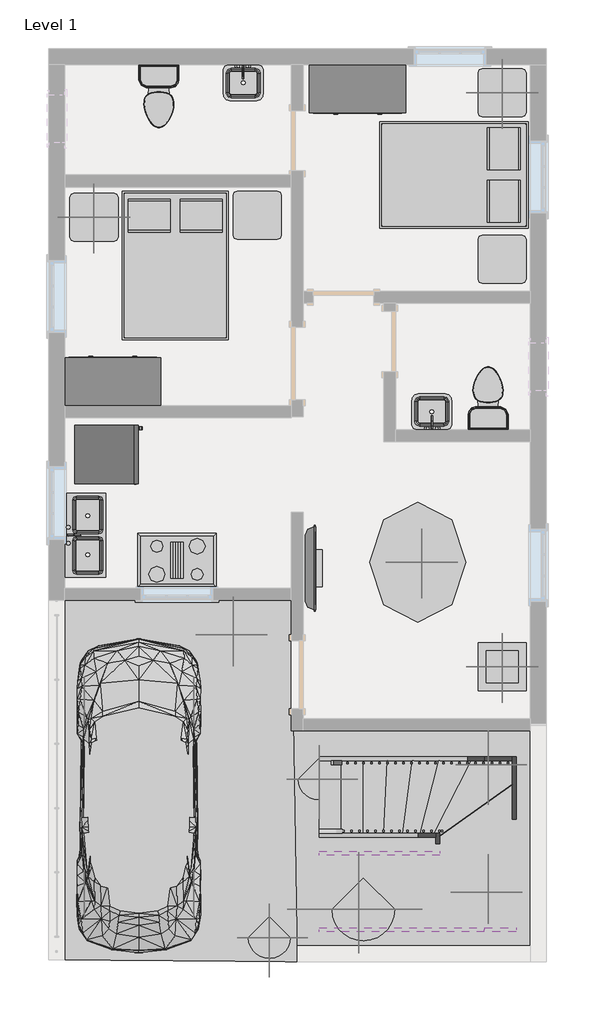
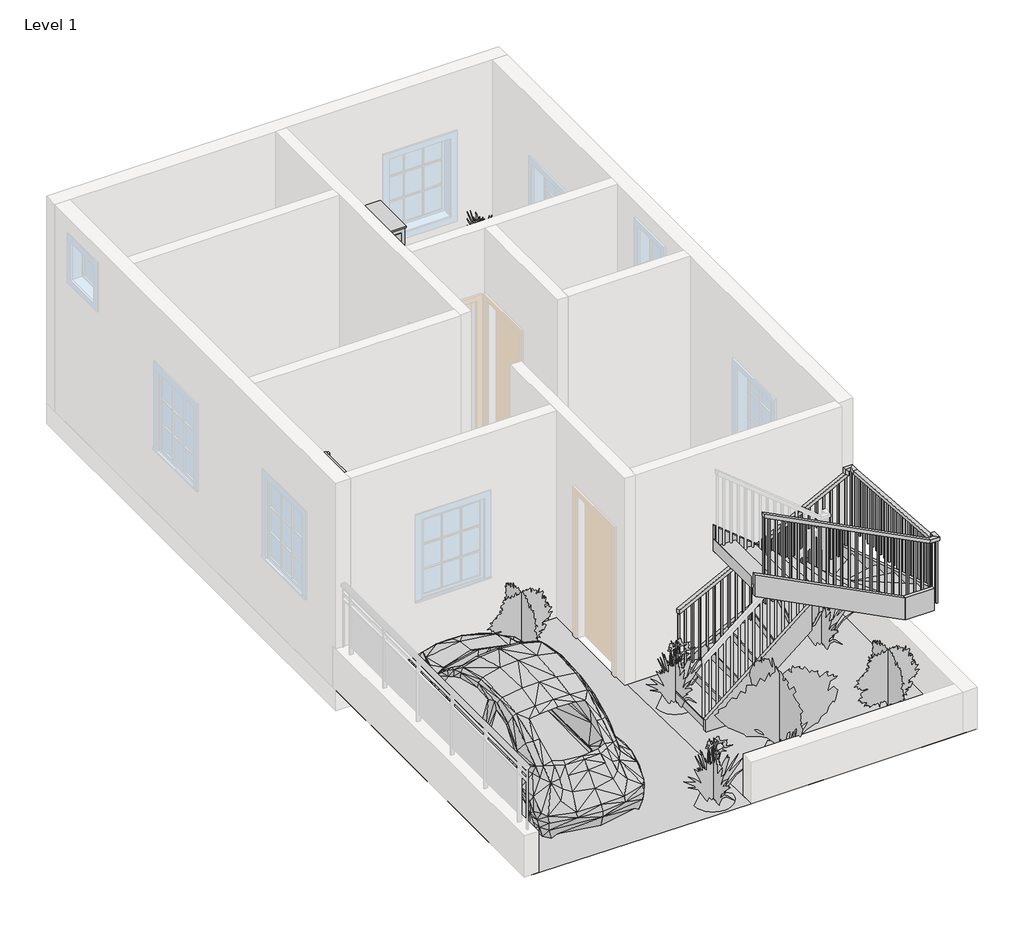
# One storey, part 2 of 2: 11 furniture elements, 10 geographic elements, 8 members, 7 flow terminals, 5 proxies, 1 railing, 1 stair flight.
"""IFC4 building model written with IfcOpenShell, lengths in millimetres."""

from ifc_helpers import new_model, si_unit, frame, origin, place, context, project, spatial, polyline, outline, extrude, faceted_brep, triangles, transform, mapped, element, save
from components import proxy_bb1e6e30, rpc_beetle_rpc_beetle_3ce7ba48, proxy_a13a33b2, flow_terminal_accce45a, flow_terminal_a53be723, flow_terminal_62a433f7, toilet_domestic_3d_toilet_domestic_3d_f7549cf7, toilet_domestic_3d_toilet_domestic_3d_183bbd19, furniture_c8abb964, furniture_2babcf72, furniture_7a3aaa4f, furniture_b5c51a22, furniture_743965d2, furniture_31d08a24, rpc_plant_tropical_55f6ff97, rpc_plant_tropical_6475341c, rpc_plant_tropical_agave_1_5_93a2a214, rpc_plant_tropical_jungle_flame_3_9c4808c2, stair_flight_9cd34823

model = new_model("IFC4")

# Units and contexts
model_context = context("Model", 3, world=origin())
ifc_project = project(units=[si_unit("LENGTHUNIT", "METRE", prefix="MILLI")], contexts=[model_context])

# Site, building, storey
site = spatial("IfcSite", under=ifc_project)
building = spatial("IfcBuilding", under=site)
storey = spatial("IfcBuildingStorey", under=building, Name="Level 1", Elevation=0.0)

# Proxies
placement = place(None, origin())
element("IfcBuildingElementProxy", 1, Name="Building Element Proxy", at=placement, inside=storey, context=model_context, shape_type="Tessellation", body=[
    triangles([(-13440.8586548, 7159.8083221, 0.0), (-10367.4590424, 7159.8083221, 0.0), (-10291.2590424, 2587.8086128, 0.0), (-13440.8586548, 2714.808419, 0.0), (-13440.8586548, 2613.2085159, 0.0)], [[4, 2, 1], [4, 3, 2], [3, 4, 5]], closed=False),
])
element("IfcBuildingElementProxy", 2, Name="Building Element Proxy", at=placement, inside=storey, context=model_context, shape_type="Tessellation", body=[
    triangles([(-7141.6588486, 5572.3087097, 0.0), (-10367.4590424, 5508.8085159, 0.0), (-10291.2590424, 2587.8086128, 0.0), (-7141.6588486, 2587.8086128, 0.0)], [[2, 3, 1], [4, 1, 3]], closed=False),
])
proxy_shape = proxy_bb1e6e30(model_context)
element("IfcBuildingElementProxy", 3, Name="Cook Top-4 Unit : 36\" x 20\"", ObjectType="Cook Top-4 Unit : 36\" x 20\"", at=placement, inside=storey, context=model_context, shape_type="MappedRepresentation", body=[
    mapped(proxy_shape, transform((-11815.2586966, 7667.8085318, 0.0), x_axis=(1.0, 0.0, 0.0), y_axis=(0.0, 1.0, 0.0), z_axis=(0.0, 0.0, 1.0))),
])
rpc_beetle_rpc_beetle_shape = rpc_beetle_rpc_beetle_3ce7ba48(model_context)
element("IfcBuildingElementProxy", 4, Name="RPC Beetle : RPC Beetle", ObjectType="RPC Beetle : RPC Beetle", at=placement, inside=storey, context=model_context, shape_type="MappedRepresentation", body=[
    mapped(rpc_beetle_rpc_beetle_shape, transform((-12297.8586966, 3451.4085318, 0.0), x_axis=(1.0, 0.0, 0.0), y_axis=(0.0, 1.0, 0.0), z_axis=(0.0, 0.0, 1.0))),
])
proxy_2_shape = proxy_a13a33b2(model_context)
element("IfcBuildingElementProxy", 5, Name="Refrigerator : 30\" x 32\" RH", ObjectType="Refrigerator : 30\" x 32\" RH", at=placement, inside=storey, context=model_context, shape_type="MappedRepresentation", body=[
    mapped(proxy_2_shape, transform((-12721.7211966, 9006.4595603, 0.0), x_axis=(0.0, 1.0000000000000002, 0.0), y_axis=(-1.0000000000000002, 0.0, 0.0), z_axis=(0.0, 0.0, 1.0))),
])

# Flow terminals
flow_terminal_shape = flow_terminal_accce45a(model_context)
element("IfcFlowTerminal", 6, ObjectType="Floor Drain - Round : 5\" Strainer - 2\" Drain", at=placement, inside=storey, context=model_context, shape_type="MappedRepresentation", body=[
    mapped(flow_terminal_shape, transform((-12907.4586966, 13738.4085318, 0.0), x_axis=(1.0, 0.0, 0.0), y_axis=(0.0, 1.0, 0.0), z_axis=(0.0, 0.0, 1.0))),
])
element("IfcFlowTerminal", 7, ObjectType="Floor Drain - Round : 5\" Strainer - 2\" Drain", at=placement, inside=storey, context=model_context, shape_type="MappedRepresentation", body=[
    mapped(flow_terminal_shape, transform((-7700.4586966, 10766.6085318, 0.0), x_axis=(1.0, 0.0, 0.0), y_axis=(0.0, 1.0, 0.0), z_axis=(0.0, 0.0, 1.0))),
])
flow_terminal_2_shape = flow_terminal_a53be723(model_context)
element("IfcFlowTerminal", 8, ObjectType="Sink Kitchen-Double : 42\" x 21\"", at=placement, inside=storey, context=model_context, shape_type="MappedRepresentation", body=[
    mapped(flow_terminal_2_shape, transform((-12981.3132954, 7969.6192912, 0.0), x_axis=(0.0, 1.0000000000000002, 0.0), y_axis=(-1.0000000000000002, 0.0, 0.0), z_axis=(0.0, 0.0, 1.0))),
])
flow_terminal_3_shape = flow_terminal_62a433f7(model_context)
element("IfcFlowTerminal", 9, ObjectType="Sink Vanity-Square : 20\" x 18\"", at=placement, inside=storey, context=model_context, shape_type="MappedRepresentation", body=[
    mapped(flow_terminal_3_shape, transform((-10992.7479371, 13761.4631306, 0.0), x_axis=(1.0, 0.0, 0.0), y_axis=(0.0, 1.0, 0.0), z_axis=(0.0, 0.0, 1.0))),
])
element("IfcFlowTerminal", 10, ObjectType="Sink Vanity-Square : 20\" x 18\"", at=placement, inside=storey, context=model_context, shape_type="MappedRepresentation", body=[
    mapped(flow_terminal_3_shape, transform((-8573.769456, 9498.9539329, 0.0), x_axis=(-1.0, 0.0, 0.0), y_axis=(0.0, -1.0, 0.0), z_axis=(0.0, 0.0, 1.0))),
])
toilet_domestic_3d_toilet_domestic_3d_shape = toilet_domestic_3d_toilet_domestic_3d_f7549cf7(model_context)
toilet_domestic_3d_toilet_domestic_3d_2_shape = toilet_domestic_3d_toilet_domestic_3d_183bbd19(model_context)
element("IfcFlowTerminal", 11, ObjectType="Toilet-Domestic-3D : Toilet-Domestic-3D", at=placement, inside=storey, context=model_context, shape_type="MappedRepresentation", body=[
    mapped(toilet_domestic_3d_toilet_domestic_3d_shape, transform((-12043.8586966, 13446.9125044, 0.0), x_axis=(1.0, 0.0, 0.0), y_axis=(0.0, 1.0, 0.0), z_axis=(0.0, 0.0, 1.0))),
    mapped(toilet_domestic_3d_toilet_domestic_3d_2_shape, transform((-12043.8586966, 13446.9125044, 0.0), x_axis=(1.0, 0.0, 0.0), y_axis=(0.0, 1.0, 0.0), z_axis=(0.0, 0.0, 1.0))),
])
element("IfcFlowTerminal", 12, ObjectType="Toilet-Domestic-3D : Toilet-Domestic-3D", at=placement, inside=storey, context=model_context, shape_type="MappedRepresentation", body=[
    mapped(toilet_domestic_3d_toilet_domestic_3d_shape, transform((-7878.2586966, 9813.5045591, 0.0), x_axis=(-1.0, 0.0, 0.0), y_axis=(0.0, -1.0, 0.0), z_axis=(0.0, 0.0, 1.0))),
    mapped(toilet_domestic_3d_toilet_domestic_3d_2_shape, transform((-7878.2586966, 9813.5045591, 0.0), x_axis=(-1.0, 0.0, 0.0), y_axis=(0.0, -1.0, 0.0), z_axis=(0.0, 0.0, 1.0))),
])

# Furniture
furniture_shape = furniture_c8abb964(model_context)
element("IfcFurniture", 13, ObjectType="Bed-Box : Double 53\" x 74\"", at=placement, inside=storey, context=model_context, shape_type="MappedRepresentation", body=[
    mapped(furniture_shape, transform((-8075.6291884, 12883.7609908, 0.0), x_axis=(0.0, -1.0000000000000004, 0.0), y_axis=(1.0000000000000004, 0.0, 0.0), z_axis=(0.0, 0.0, 1.0))),
])
element("IfcFurniture", 14, ObjectType="Bed-Box : Double 53\" x 74\"", at=placement, inside=storey, context=model_context, shape_type="MappedRepresentation", body=[
    mapped(furniture_shape, transform((-12176.6882047, 11633.9560727, 0.0), x_axis=(1.0000000000000007, 0.0, 0.0), y_axis=(0.0, 1.0000000000000007, 0.0), z_axis=(0.0, 0.0, 1.0))),
])
furniture_2_shape = furniture_2babcf72(model_context)
element("IfcFurniture", 15, ObjectType="Dresser : 48\" x 60\" x 24\"", at=placement, inside=storey, context=model_context, shape_type="MappedRepresentation", body=[
    mapped(furniture_2_shape, transform((-9260.0654367, 13999.9714858, 0.0), x_axis=(1.0, 0.0, 0.0), y_axis=(0.0, 1.0, 0.0), z_axis=(0.0, 0.0, 1.0))),
])
element("IfcFurniture", 16, ObjectType="Dresser : 48\" x 60\" x 24\"", at=placement, inside=storey, context=model_context, shape_type="MappedRepresentation", body=[
    mapped(furniture_2_shape, transform((-12897.2519564, 9565.2455777, 0.0), x_axis=(-1.0000000000000004, 0.0, 0.0), y_axis=(0.0, -1.0000000000000004, 0.0), z_axis=(0.0, 0.0, 1.0))),
])
furniture_3_shape = furniture_7a3aaa4f(model_context)
element("IfcFurniture", 17, ObjectType="TV - Flat Screen : 42\"", at=placement, inside=storey, context=model_context, shape_type="MappedRepresentation", body=[
    mapped(furniture_3_shape, transform((-10131.1200729, 7570.1530459, 914.4), x_axis=(0.0, 1.0, 0.0), y_axis=(-1.0, 0.0, 0.0), z_axis=(0.0, 0.0, 1.0))),
])
furniture_4_shape = furniture_b5c51a22(model_context)
element("IfcFurniture", 18, ObjectType="Table-Coffee : 24\" x 24\" x 24\"", at=placement, inside=storey, context=model_context, shape_type="MappedRepresentation", body=[
    mapped(furniture_4_shape, transform((-7718.7244632, 6226.3974539, 0.0), x_axis=(1.0, 0.0, 0.0), y_axis=(0.0, 1.0, 0.0), z_axis=(0.0, 0.0, 1.0))),
])
furniture_5_shape = furniture_743965d2(model_context)
element("IfcFurniture", 19, ObjectType="Table-Ellipse : 60\" x 48\"", at=placement, inside=storey, context=model_context, shape_type="MappedRepresentation", body=[
    mapped(furniture_5_shape, transform((-8767.2586966, 7642.4085318, 0.0), x_axis=(0.0, 1.0000000000000002, 0.0), y_axis=(-1.0000000000000002, 0.0, 0.0), z_axis=(0.0, 0.0, 1.0))),
])
furniture_6_shape = furniture_31d08a24(model_context)
element("IfcFurniture", 20, ObjectType="Table-End : 24\" x 24\"", at=placement, inside=storey, context=model_context, shape_type="MappedRepresentation", body=[
    mapped(furniture_6_shape, transform((-8008.9923268, 13433.6085318, 0.0), x_axis=(1.0, 0.0, 0.0), y_axis=(0.0, 1.0, 0.0), z_axis=(0.0, 0.0, 1.0))),
])
element("IfcFurniture", 21, ObjectType="Table-End : 24\" x 24\"", at=placement, inside=storey, context=model_context, shape_type="MappedRepresentation", body=[
    mapped(furniture_6_shape, transform((-8008.9923268, 11325.4085318, 0.0), x_axis=(1.0, 0.0, 0.0), y_axis=(0.0, 1.0, 0.0), z_axis=(0.0, 0.0, 1.0))),
])
element("IfcFurniture", 22, ObjectType="Table-End : 24\" x 24\"", at=placement, inside=storey, context=model_context, shape_type="MappedRepresentation", body=[
    mapped(furniture_6_shape, transform((-11107.7923268, 11882.1265645, 0.0), x_axis=(1.0, 0.0, 0.0), y_axis=(0.0, 1.0, 0.0), z_axis=(0.0, 0.0, 1.0))),
])
element("IfcFurniture", 23, ObjectType="Table-End : 24\" x 24\"", at=placement, inside=storey, context=model_context, shape_type="MappedRepresentation", body=[
    mapped(furniture_6_shape, transform((-13174.769376, 11856.7265645, 0.0), x_axis=(1.0, 0.0, 0.0), y_axis=(0.0, 1.0, 0.0), z_axis=(0.0, 0.0, 1.0))),
])

# Geographic elements
rpc_plant_tropical_shape = rpc_plant_tropical_55f6ff97(model_context)
element("IfcGeographicElement", 24, ObjectType="RPC Plant - Tropical", at=placement, inside=storey, context=model_context, shape_type="MappedRepresentation", body=[
    mapped(rpc_plant_tropical_shape, transform((-10646.8586966, 2892.6085318, 0.0), x_axis=(1.0, 0.0, 0.0), y_axis=(0.0, 1.0, 0.0), z_axis=(0.0, 0.0, 1.0))),
])
element("IfcGeographicElement", 25, ObjectType="RPC Plant - Tropical", at=placement, inside=storey, context=model_context, shape_type="MappedRepresentation", body=[
    mapped(rpc_plant_tropical_shape, transform((-7878.2586966, 5077.0085318, 0.0), x_axis=(1.0, 0.0, 0.0), y_axis=(0.0, 1.0, 0.0), z_axis=(0.0, 0.0, 1.0))),
])
element("IfcGeographicElement", 26, ObjectType="RPC Plant - Tropical", at=placement, inside=storey, context=model_context, shape_type="MappedRepresentation", body=[
    mapped(rpc_plant_tropical_shape, transform((-10015.5903884, 4899.2085318, 0.0), x_axis=(1.0, 0.0, 0.0), y_axis=(0.0, 1.0, 0.0), z_axis=(0.0, 0.0, 1.0))),
])
rpc_plant_tropical_2_shape = rpc_plant_tropical_6475341c(model_context)
element("IfcGeographicElement", 27, ObjectType="RPC Plant - Tropical", at=placement, inside=storey, context=model_context, shape_type="MappedRepresentation", body=[
    mapped(rpc_plant_tropical_2_shape, transform((-9456.7903884, 3248.2085318, 0.0), x_axis=(1.0, 0.0, 0.0), y_axis=(0.0, 1.0, 0.0), z_axis=(0.0, 0.0, 1.0))),
])
rpc_plant_tropical_agave_1_5_shape = rpc_plant_tropical_agave_1_5_93a2a214(model_context)
element("IfcGeographicElement", 28, ObjectType="RPC Plant - Tropical : Agave - 1.5'", at=placement, inside=storey, context=model_context, shape_type="MappedRepresentation", body=[
    mapped(rpc_plant_tropical_agave_1_5_shape, transform((-7700.4586966, 13586.0085318, 609.6), x_axis=(1.0, 0.0, 0.0), y_axis=(0.0, 1.0, 0.0), z_axis=(0.0, 0.0, 1.0))),
])
element("IfcGeographicElement", 29, ObjectType="RPC Plant - Tropical : Agave - 1.5'", at=placement, inside=storey, context=model_context, shape_type="MappedRepresentation", body=[
    mapped(rpc_plant_tropical_agave_1_5_shape, transform((-12866.2357457, 12009.1265645, 609.6), x_axis=(1.0, 0.0, 0.0), y_axis=(0.0, 1.0, 0.0), z_axis=(0.0, 0.0, 1.0))),
])
element("IfcGeographicElement", 30, ObjectType="RPC Plant - Tropical : Agave - 1.5'", at=placement, inside=storey, context=model_context, shape_type="MappedRepresentation", body=[
    mapped(rpc_plant_tropical_agave_1_5_shape, transform((-7700.4586966, 6321.6085318, 609.6), x_axis=(1.0, 0.0, 0.0), y_axis=(0.0, 1.0, 0.0), z_axis=(0.0, 0.0, 1.0))),
])
element("IfcGeographicElement", 31, ObjectType="RPC Plant - Tropical : Agave - 1.5'", at=placement, inside=storey, context=model_context, shape_type="MappedRepresentation", body=[
    mapped(rpc_plant_tropical_agave_1_5_shape, transform((-8716.4586966, 7642.4085318, 762.0), x_axis=(1.0, 0.0, 0.0), y_axis=(0.0, 1.0, 0.0), z_axis=(0.0, 0.0, 1.0))),
])
rpc_plant_tropical_jungle_flame_3_shape = rpc_plant_tropical_jungle_flame_3_9c4808c2(model_context)
element("IfcGeographicElement", 32, ObjectType="RPC Plant - Tropical : Jungle Flame - 3'", at=placement, inside=storey, context=model_context, shape_type="MappedRepresentation", body=[
    mapped(rpc_plant_tropical_jungle_flame_3_shape, transform((-11104.0586966, 6728.0085318, 0.0), x_axis=(1.0, 0.0, 0.0), y_axis=(0.0, 1.0, 0.0), z_axis=(0.0, 0.0, 1.0))),
])
element("IfcGeographicElement", 33, ObjectType="RPC Plant - Tropical : Jungle Flame - 3'", at=placement, inside=storey, context=model_context, shape_type="MappedRepresentation", body=[
    mapped(rpc_plant_tropical_jungle_flame_3_shape, transform((-7878.2586966, 3467.7118501, 0.0), x_axis=(1.0, 0.0, 0.0), y_axis=(0.0, 1.0, 0.0), z_axis=(0.0, 0.0, 1.0))),
])

# Members
element("IfcMember", 34, ObjectType="Stringer - 2\" Width", at=placement, inside=storey, context=model_context, shape_type="SweptSolid", body=[
    extrude(outline(polyline([(229.639954, -10015.5903884), (0.0, -10015.5903884), (0.0, -9795.8280709), (962.500629, -7928.1731967), (1305.3956453, -7928.1731967), (229.639954, -10015.5903884)])), frame((0.0, 5127.8085318, 0.0), z_axis=(0.0, 1.0, 0.0), x_axis=(0.0, 0.0, 1.0)), (0.0, 0.0, 1.0), 50.8),
])
element("IfcMember", 35, ObjectType="Stringer - 2\" Width", at=placement, inside=storey, context=model_context, shape_type="SweptSolid", body=[
    extrude(outline(polyline([(-7928.1731967, 5127.8085318), (-7928.1731967, 5178.6085318), (-7573.4586966, 5178.6085318), (-7573.4586966, 5127.8085318), (-7928.1731967, 5127.8085318)])), frame((0.0, 0.0, 962.500629), z_axis=(0.0, 0.0, 1.0), x_axis=(1.0, 0.0, 0.0)), (0.0, 0.0, 1.0), 342.8950162),
])
element("IfcMember", 36, ObjectType="Stringer - 2\" Width", at=placement, inside=storey, context=model_context, shape_type="SweptSolid", body=[
    extrude(outline(polyline([(5178.6085318, 1289.0952212), (5178.6085318, 1000.5956453), (5009.0860488, 1000.5956453), (3019.6085318, 1638.9682298), (3019.6085318, 1969.9972697), (3056.588649, 1969.9972697), (5178.6085318, 1289.0952212)])), frame((-7573.4586966, 0.0, 0.0), z_axis=(1.0, 0.0, 0.0), x_axis=(0.0, 1.0, 0.0)), (0.0, 0.0, 1.0), 50.8),
])
element("IfcMember", 37, ObjectType="Stringer - 2\" Width", at=placement, inside=storey, context=model_context, shape_type="SweptSolid", body=[
    extrude(outline(polyline([(-7522.6586966, 3019.6085318), (-7522.6586966, 2968.8085318), (-7928.1731967, 2968.8085318), (-7928.1731967, 3019.6085318), (-7522.6586966, 3019.6085318)])), frame((0.0, 0.0, 1649.8904473), z_axis=(0.0, 0.0, 1.0), x_axis=(1.0, 0.0, 0.0)), (0.0, 0.0, 1.0), 320.1068224),
])
element("IfcMember", 38, ObjectType="Stringer - 2\" Width", at=placement, inside=storey, context=model_context, shape_type="SweptSolid", body=[
    extrude(outline(polyline([(1649.8904473, -7928.1731967), (1969.9972697, -7928.1731967), (3045.7529609, -10015.5903884), (2725.6461385, -10015.5903884), (1649.8904473, -7928.1731967)])), frame((0.0, 2968.8085318, 0.0), z_axis=(0.0, 1.0, 0.0), x_axis=(0.0, 0.0, 1.0)), (0.0, 0.0, 1.0), 50.8),
])
element("IfcMember", 39, ObjectType="Stringer - 2\" Width", at=placement, inside=storey, context=model_context, shape_type="SweptSolid", body=[
    extrude(outline(polyline([(176.1764461, -10015.5903884), (0.0, -10015.5903884), (0.0, -9749.3287439), (987.1410923, -8538.6586966), (1380.418648, -8538.6586966), (176.1764461, -10015.5903884)])), frame((0.0, 4162.6085318, 0.0), z_axis=(0.0, 1.0, 0.0), x_axis=(0.0, 0.0, 1.0)), (0.0, 0.0, 1.0), 50.8),
])
element("IfcMember", 40, ObjectType="Stringer - 2\" Width", at=placement, inside=storey, context=model_context, shape_type="SweptSolid", body=[
    extrude(outline(polyline([(4213.4085318, 1573.2682978), (4213.4085318, 1028.5617647), (4179.1663144, 1028.5617647), (3984.8085318, 1360.465107), (3984.8085318, 1926.1409689), (4006.7714143, 1926.1409689), (4213.4085318, 1573.2682978)])), frame((-8538.6586966, 0.0, 0.0), z_axis=(1.0, 0.0, 0.0), x_axis=(0.0, 1.0, 0.0)), (0.0, 0.0, 1.0), 50.8),
])
element("IfcMember", 41, ObjectType="Stringer - 2\" Width", at=placement, inside=storey, context=model_context, shape_type="SweptSolid", body=[
    extrude(outline(polyline([(1532.8634131, -8487.8586966), (1926.1409689, -8487.8586966), (3171.8038432, -10015.5903884), (2778.5262875, -10015.5903884), (1532.8634131, -8487.8586966)])), frame((0.0, 3934.0085318, 0.0), z_axis=(0.0, 1.0, 0.0), x_axis=(0.0, 0.0, 1.0)), (0.0, 0.0, 1.0), 50.8),
])

# Railing
element("IfcRailing", 42, ObjectType="Handrail - Rectangular", at=placement, inside=storey, context=model_context, shape_type="SolidModel", body=[
    faceted_brep([(-9863.1903884, 5127.8085318, 1187.6168978), (-9863.1903884, 5127.8085318, 1130.4677284), (-9863.1903884, 5077.0085318, 1130.4677284), (-9863.1903884, 5077.0085318, 1187.6168978), (-7548.0586966, 5127.8085318, 2380.7258284), (-7497.2586966, 5127.8085318, 2349.7565666), (-7497.2586966, 5077.0085318, 2349.7565666), (-7548.0586966, 5077.0085318, 2380.7258284), (-7421.0586966, 4998.958193, 2404.6395816), (-7421.0586966, 5000.8085318, 2455.4395816), (-7421.0586966, 3146.6085318, 2590.6937517), (-7421.0586966, 3095.8085318, 2543.4643729), (-7471.8586966, 4998.958193, 2404.6395816), (-7471.8586966, 3095.8085318, 2543.4643729), (-7471.8586966, 5000.8085318, 2455.4395816), (-7471.8586966, 3146.6085318, 2590.6937517), (-9863.1903884, 3019.6085318, 3858.5164356), (-9863.1903884, 3070.4085318, 3858.5164356), (-9863.1903884, 3070.4085318, 3801.3672662), (-9863.1903884, 3019.6085318, 3801.3672662), (-7560.3787478, 3019.6085318, 2614.6075049), (-7548.0586966, 3019.6085318, 2665.4075049), (-7560.3787478, 3070.4085318, 2614.6075049), (-7548.0586966, 3070.4085318, 2665.4075049), (-7548.0586966, 5127.8085318, 2455.4395816), (-7497.2586966, 5127.8085318, 2404.6395816), (-7497.2586966, 5077.0085318, 2404.6395816), (-7548.0586966, 5077.0085318, 2455.4395816), (-7421.0586966, 5127.8085318, 2455.4395816), (-7421.0586966, 5127.8085318, 2404.6395816), (-7471.8586966, 5077.0085318, 2404.6395816), (-7471.8586966, 5077.0085318, 2455.4395816), (-7421.0586966, 3146.6085318, 2665.4075049), (-7421.0586966, 3095.8085318, 2614.6075049), (-7471.8586966, 3095.8085318, 2614.6075049), (-7471.8586966, 3146.6085318, 2665.4075049), (-7421.0586966, 3019.6085318, 2665.4075049), (-7421.0586966, 3019.6085318, 2614.6075049), (-7471.8586966, 3070.4085318, 2614.6075049), (-7471.8586966, 3070.4085318, 2665.4075049)], [[[0, 1, 2, 3]], [[1, 0, 4, 5]], [[2, 1, 5, 6]], [[3, 2, 6, 7]], [[0, 3, 7, 4]], [[8, 9, 10, 11]], [[12, 8, 11, 13]], [[14, 12, 13, 15]], [[9, 14, 15, 10]], [[16, 17, 18, 19]], [[20, 21, 16, 19]], [[22, 20, 19, 18]], [[23, 22, 18, 17]], [[21, 23, 17, 16]], [[5, 4, 24, 25]], [[6, 5, 25, 26]], [[7, 6, 26, 27]], [[4, 7, 27, 24]], [[25, 24, 28, 29]], [[26, 25, 29, 30]], [[27, 26, 30, 31]], [[24, 27, 31, 28]], [[29, 28, 9, 8]], [[30, 29, 8, 12]], [[31, 30, 12, 14]], [[28, 31, 14, 9]], [[11, 10, 32, 33]], [[13, 11, 33, 34]], [[15, 13, 34, 35]], [[10, 15, 35, 32]], [[33, 32, 36, 37]], [[34, 33, 37, 38]], [[35, 34, 38, 39]], [[32, 35, 39, 36]], [[37, 36, 21, 20]], [[38, 37, 20, 22]], [[39, 38, 22, 23]], [[36, 39, 23, 21]]]),
    extrude(outline(polyline([(3765.0830008, -9792.7836966), (2878.6666667, -9792.7836966), (2878.6666667, -9773.7336966), (3755.2655354, -9773.7336966), (3765.0830008, -9792.7836966)])), frame((0.0, 3035.4835318, 0.0), z_axis=(0.0, 1.0, 0.0), x_axis=(0.0, 0.0, 1.0)), (0.0, 0.0, 1.0), 19.05),
    extrude(outline(polyline([(3712.7231856, -9691.1836966), (2709.3333333, -9691.1836966), (2709.3333333, -9672.1336966), (3702.9057203, -9672.1336966), (3712.7231856, -9691.1836966)])), frame((0.0, 3035.4835318, 0.0), z_axis=(0.0, 1.0, 0.0), x_axis=(0.0, 0.0, 1.0)), (0.0, 0.0, 1.0), 19.05),
    extrude(outline(polyline([(3660.3633705, -9589.5836966), (2709.3333333, -9589.5836966), (2709.3333333, -9570.5336966), (3650.5459052, -9570.5336966), (3660.3633705, -9589.5836966)])), frame((0.0, 3035.4835318, 0.0), z_axis=(0.0, 1.0, 0.0), x_axis=(0.0, 0.0, 1.0)), (0.0, 0.0, 1.0), 19.05),
    extrude(outline(polyline([(3608.0035554, -9487.9836966), (2709.3333333, -9487.9836966), (2709.3333333, -9468.9336966), (3598.1860901, -9468.9336966), (3608.0035554, -9487.9836966)])), frame((0.0, 3035.4835318, 0.0), z_axis=(0.0, 1.0, 0.0), x_axis=(0.0, 0.0, 1.0)), (0.0, 0.0, 1.0), 19.05),
    extrude(outline(polyline([(3555.6437403, -9386.3836966), (2540.0, -9386.3836966), (2540.0, -9367.3336966), (3545.826275, -9367.3336966), (3555.6437403, -9386.3836966)])), frame((0.0, 3035.4835318, 0.0), z_axis=(0.0, 1.0, 0.0), x_axis=(0.0, 0.0, 1.0)), (0.0, 0.0, 1.0), 19.05),
    extrude(outline(polyline([(3503.2839252, -9284.7836966), (2540.0, -9284.7836966), (2540.0, -9265.7336966), (3493.4664598, -9265.7336966), (3503.2839252, -9284.7836966)])), frame((0.0, 3035.4835318, 0.0), z_axis=(0.0, 1.0, 0.0), x_axis=(0.0, 0.0, 1.0)), (0.0, 0.0, 1.0), 19.05),
    extrude(outline(polyline([(3450.9241101, -9183.1836966), (2540.0, -9183.1836966), (2540.0, -9164.1336966), (3441.1066447, -9164.1336966), (3450.9241101, -9183.1836966)])), frame((0.0, 3035.4835318, 0.0), z_axis=(0.0, 1.0, 0.0), x_axis=(0.0, 0.0, 1.0)), (0.0, 0.0, 1.0), 19.05),
    extrude(outline(polyline([(3398.5642949, -9081.5836966), (2370.6666667, -9081.5836966), (2370.6666667, -9062.5336966), (3388.7468296, -9062.5336966), (3398.5642949, -9081.5836966)])), frame((0.0, 3035.4835318, 0.0), z_axis=(0.0, 1.0, 0.0), x_axis=(0.0, 0.0, 1.0)), (0.0, 0.0, 1.0), 19.05),
    extrude(outline(polyline([(3346.2044798, -8979.9836966), (2370.6666667, -8979.9836966), (2370.6666667, -8960.9336966), (3336.3870145, -8960.9336966), (3346.2044798, -8979.9836966)])), frame((0.0, 3035.4835318, 0.0), z_axis=(0.0, 1.0, 0.0), x_axis=(0.0, 0.0, 1.0)), (0.0, 0.0, 1.0), 19.05),
    extrude(outline(polyline([(3293.8446647, -8878.3836966), (2370.6666667, -8878.3836966), (2370.6666667, -8859.3336966), (3284.0271994, -8859.3336966), (3293.8446647, -8878.3836966)])), frame((0.0, 3035.4835318, 0.0), z_axis=(0.0, 1.0, 0.0), x_axis=(0.0, 0.0, 1.0)), (0.0, 0.0, 1.0), 19.05),
    extrude(outline(polyline([(3241.4848496, -8776.7836966), (2201.3333333, -8776.7836966), (2201.3333333, -8757.7336966), (3231.6673843, -8757.7336966), (3241.4848496, -8776.7836966)])), frame((0.0, 3035.4835318, 0.0), z_axis=(0.0, 1.0, 0.0), x_axis=(0.0, 0.0, 1.0)), (0.0, 0.0, 1.0), 19.05),
    extrude(outline(polyline([(3189.1250345, -8675.1836966), (2201.3333333, -8675.1836966), (2201.3333333, -8656.1336966), (3179.3075691, -8656.1336966), (3189.1250345, -8675.1836966)])), frame((0.0, 3035.4835318, 0.0), z_axis=(0.0, 1.0, 0.0), x_axis=(0.0, 0.0, 1.0)), (0.0, 0.0, 1.0), 19.05),
    extrude(outline(polyline([(3136.7652194, -8573.5836966), (2201.3333333, -8573.5836966), (2201.3333333, -8554.5336966), (3126.947754, -8554.5336966), (3136.7652194, -8573.5836966)])), frame((0.0, 3035.4835318, 0.0), z_axis=(0.0, 1.0, 0.0), x_axis=(0.0, 0.0, 1.0)), (0.0, 0.0, 1.0), 19.05),
    extrude(outline(polyline([(3084.4054042, -8471.9836966), (2032.0, -8471.9836966), (2032.0, -8452.9336966), (3074.5879389, -8452.9336966), (3084.4054042, -8471.9836966)])), frame((0.0, 3035.4835318, 0.0), z_axis=(0.0, 1.0, 0.0), x_axis=(0.0, 0.0, 1.0)), (0.0, 0.0, 1.0), 19.05),
    extrude(outline(polyline([(3032.0455891, -8370.3836966), (2032.0, -8370.3836966), (2032.0, -8351.3336966), (3022.2281238, -8351.3336966), (3032.0455891, -8370.3836966)])), frame((0.0, 3035.4835318, 0.0), z_axis=(0.0, 1.0, 0.0), x_axis=(0.0, 0.0, 1.0)), (0.0, 0.0, 1.0), 19.05),
    extrude(outline(polyline([(2979.685774, -8268.7836966), (2032.0, -8268.7836966), (2032.0, -8249.7336966), (2969.8683087, -8249.7336966), (2979.685774, -8268.7836966)])), frame((0.0, 3035.4835318, 0.0), z_axis=(0.0, 1.0, 0.0), x_axis=(0.0, 0.0, 1.0)), (0.0, 0.0, 1.0), 19.05),
    extrude(outline(polyline([(2927.3259589, -8167.1836966), (2032.0, -8167.1836966), (2032.0, -8148.1336966), (2917.5084936, -8148.1336966), (2927.3259589, -8167.1836966)])), frame((0.0, 3035.4835318, 0.0), z_axis=(0.0, 1.0, 0.0), x_axis=(0.0, 0.0, 1.0)), (0.0, 0.0, 1.0), 19.05),
    extrude(outline(polyline([(2874.9661438, -8065.5836966), (1862.6666667, -8065.5836966), (1862.6666667, -8046.5336966), (2865.1486784, -8046.5336966), (2874.9661438, -8065.5836966)])), frame((0.0, 3035.4835318, 0.0), z_axis=(0.0, 1.0, 0.0), x_axis=(0.0, 0.0, 1.0)), (0.0, 0.0, 1.0), 19.05),
    extrude(outline(polyline([(2822.6063287, -7963.9836966), (1862.6666667, -7963.9836966), (1862.6666667, -7944.9336966), (2812.7888633, -7944.9336966), (2822.6063287, -7963.9836966)])), frame((0.0, 3035.4835318, 0.0), z_axis=(0.0, 1.0, 0.0), x_axis=(0.0, 0.0, 1.0)), (0.0, 0.0, 1.0), 19.05),
    extrude(outline(polyline([(2770.2465135, -7862.3836966), (1862.6666667, -7862.3836966), (1862.6666667, -7843.3336966), (2760.4290482, -7843.3336966), (2770.2465135, -7862.3836966)])), frame((0.0, 3035.4835318, 0.0), z_axis=(0.0, 1.0, 0.0), x_axis=(0.0, 0.0, 1.0)), (0.0, 0.0, 1.0), 19.05),
    extrude(outline(polyline([(2717.8866984, -7760.7836966), (1862.6666667, -7760.7836966), (1862.6666667, -7741.7336966), (2708.0692331, -7741.7336966), (2717.8866984, -7760.7836966)])), frame((0.0, 3035.4835318, 0.0), z_axis=(0.0, 1.0, 0.0), x_axis=(0.0, 0.0, 1.0)), (0.0, 0.0, 1.0), 19.05),
    extrude(outline(polyline([(2665.5268833, -7659.1836966), (1862.6666667, -7659.1836966), (1862.6666667, -7640.1336966), (2655.709418, -7640.1336966), (2665.5268833, -7659.1836966)])), frame((0.0, 3035.4835318, 0.0), z_axis=(0.0, 1.0, 0.0), x_axis=(0.0, 0.0, 1.0)), (0.0, 0.0, 1.0), 19.05),
    extrude(outline(polyline([(-7538.5336966, 3035.4835318), (-7557.5836966, 3035.4835318), (-7557.5836966, 3054.5335318), (-7538.5336966, 3054.5335318), (-7538.5336966, 3035.4835318)])), frame((0.0, 0.0, 1969.9972697), z_axis=(0.0, 0.0, 1.0), x_axis=(1.0, 0.0, 0.0)), (0.0, 0.0, 1.0), 644.6102352),
    extrude(outline(polyline([(-7436.9336966, 3079.9335318), (-7436.9336966, 3060.8835318), (-7455.9836966, 3060.8835318), (-7455.9836966, 3079.9335318), (-7436.9336966, 3079.9335318)])), frame((0.0, 0.0, 1681.8521423), z_axis=(0.0, 0.0, 1.0), x_axis=(1.0, 0.0, 0.0)), (0.0, 0.0, 1.0), 932.7553626),
    extrude(outline(polyline([(3181.5335318, 2537.2111836), (3181.5335318, 1674.4409549), (3162.4835318, 1674.4409549), (3162.4835318, 2538.6007812), (3181.5335318, 2537.2111836)])), frame((-7455.9836966, 0.0, 0.0), z_axis=(1.0, 0.0, 0.0), x_axis=(0.0, 1.0, 0.0)), (0.0, 0.0, 1.0), 19.05),
    extrude(outline(polyline([(3283.1335318, 2529.7999962), (3283.1335318, 1667.0297675), (3264.0835318, 1667.0297675), (3264.0835318, 2531.1895938), (3283.1335318, 2529.7999962)])), frame((-7455.9836966, 0.0, 0.0), z_axis=(1.0, 0.0, 0.0), x_axis=(0.0, 1.0, 0.0)), (0.0, 0.0, 1.0), 19.05),
    extrude(outline(polyline([(3384.7335318, 2522.3888087), (3384.7335318, 1659.6185801), (3365.6835318, 1659.6185801), (3365.6835318, 2523.7784064), (3384.7335318, 2522.3888087)])), frame((-7455.9836966, 0.0, 0.0), z_axis=(1.0, 0.0, 0.0), x_axis=(0.0, 1.0, 0.0)), (0.0, 0.0, 1.0), 19.05),
    extrude(outline(polyline([(3486.3335318, 2514.9776213), (3486.3335318, 1652.2073927), (3467.2835318, 1652.2073927), (3467.2835318, 2516.367219), (3486.3335318, 2514.9776213)])), frame((-7455.9836966, 0.0, 0.0), z_axis=(1.0, 0.0, 0.0), x_axis=(0.0, 1.0, 0.0)), (0.0, 0.0, 1.0), 19.05),
    extrude(outline(polyline([(3587.9335318, 2507.5664339), (3587.9335318, 1644.7962053), (3568.8835318, 1644.7962053), (3568.8835318, 2508.9560316), (3587.9335318, 2507.5664339)])), frame((-7455.9836966, 0.0, 0.0), z_axis=(1.0, 0.0, 0.0), x_axis=(0.0, 1.0, 0.0)), (0.0, 0.0, 1.0), 19.05),
    extrude(outline(polyline([(3689.5335318, 2500.1552465), (3689.5335318, 1637.3850179), (3670.4835318, 1637.3850179), (3670.4835318, 2501.5448442), (3689.5335318, 2500.1552465)])), frame((-7455.9836966, 0.0, 0.0), z_axis=(1.0, 0.0, 0.0), x_axis=(0.0, 1.0, 0.0)), (0.0, 0.0, 1.0), 19.05),
    extrude(outline(polyline([(3791.1335318, 2492.7440591), (3791.1335318, 1629.9738305), (3772.0835318, 1629.9738305), (3772.0835318, 2494.1336568), (3791.1335318, 2492.7440591)])), frame((-7455.9836966, 0.0, 0.0), z_axis=(1.0, 0.0, 0.0), x_axis=(0.0, 1.0, 0.0)), (0.0, 0.0, 1.0), 19.05),
    extrude(outline(polyline([(3892.7335318, 2485.3328717), (3892.7335318, 1622.5626431), (3873.6835318, 1622.5626431), (3873.6835318, 2486.7224694), (3892.7335318, 2485.3328717)])), frame((-7455.9836966, 0.0, 0.0), z_axis=(1.0, 0.0, 0.0), x_axis=(0.0, 1.0, 0.0)), (0.0, 0.0, 1.0), 19.05),
    extrude(outline(polyline([(3994.3335318, 2477.9216843), (3994.3335318, 1615.1514556), (3975.2835318, 1615.1514556), (3975.2835318, 2479.311282), (3994.3335318, 2477.9216843)])), frame((-7455.9836966, 0.0, 0.0), z_axis=(1.0, 0.0, 0.0), x_axis=(0.0, 1.0, 0.0)), (0.0, 0.0, 1.0), 19.05),
    extrude(outline(polyline([(4095.9335318, 2470.5104969), (4095.9335318, 1607.7402682), (4076.8835318, 1607.7402682), (4076.8835318, 2471.9000945), (4095.9335318, 2470.5104969)])), frame((-7455.9836966, 0.0, 0.0), z_axis=(1.0, 0.0, 0.0), x_axis=(0.0, 1.0, 0.0)), (0.0, 0.0, 1.0), 19.05),
    extrude(outline(polyline([(4197.5335318, 2463.0993095), (4197.5335318, 1600.3290808), (4178.4835318, 1600.3290808), (4178.4835318, 2464.4889071), (4197.5335318, 2463.0993095)])), frame((-7455.9836966, 0.0, 0.0), z_axis=(1.0, 0.0, 0.0), x_axis=(0.0, 1.0, 0.0)), (0.0, 0.0, 1.0), 19.05),
    extrude(outline(polyline([(4299.1335318, 2455.6881221), (4299.1335318, 1592.9178934), (4280.0835318, 1592.9178934), (4280.0835318, 2457.0777197), (4299.1335318, 2455.6881221)])), frame((-7455.9836966, 0.0, 0.0), z_axis=(1.0, 0.0, 0.0), x_axis=(0.0, 1.0, 0.0)), (0.0, 0.0, 1.0), 19.05),
    extrude(outline(polyline([(4400.7335318, 2448.2769347), (4400.7335318, 1585.506706), (4381.6835318, 1585.506706), (4381.6835318, 2449.6665323), (4400.7335318, 2448.2769347)])), frame((-7455.9836966, 0.0, 0.0), z_axis=(1.0, 0.0, 0.0), x_axis=(0.0, 1.0, 0.0)), (0.0, 0.0, 1.0), 19.05),
    extrude(outline(polyline([(4502.3335318, 2440.8657473), (4502.3335318, 1578.0955186), (4483.2835318, 1578.0955186), (4483.2835318, 2442.2553449), (4502.3335318, 2440.8657473)])), frame((-7455.9836966, 0.0, 0.0), z_axis=(1.0, 0.0, 0.0), x_axis=(0.0, 1.0, 0.0)), (0.0, 0.0, 1.0), 19.05),
    extrude(outline(polyline([(4603.9335318, 2433.4545599), (4603.9335318, 1570.6843312), (4584.8835318, 1570.6843312), (4584.8835318, 2434.8441575), (4603.9335318, 2433.4545599)])), frame((-7455.9836966, 0.0, 0.0), z_axis=(1.0, 0.0, 0.0), x_axis=(0.0, 1.0, 0.0)), (0.0, 0.0, 1.0), 19.05),
    extrude(outline(polyline([(4705.5335318, 2426.0433725), (4705.5335318, 1563.2731438), (4686.4835318, 1563.2731438), (4686.4835318, 2427.4329701), (4705.5335318, 2426.0433725)])), frame((-7455.9836966, 0.0, 0.0), z_axis=(1.0, 0.0, 0.0), x_axis=(0.0, 1.0, 0.0)), (0.0, 0.0, 1.0), 19.05),
    extrude(outline(polyline([(4807.1335318, 2418.6321851), (4807.1335318, 1555.8619564), (4788.0835318, 1555.8619564), (4788.0835318, 2420.0217827), (4807.1335318, 2418.6321851)])), frame((-7455.9836966, 0.0, 0.0), z_axis=(1.0, 0.0, 0.0), x_axis=(0.0, 1.0, 0.0)), (0.0, 0.0, 1.0), 19.05),
    extrude(outline(polyline([(4908.7335318, 2411.2209977), (4908.7335318, 1548.450769), (4889.6835318, 1548.450769), (4889.6835318, 2412.6105953), (4908.7335318, 2411.2209977)])), frame((-7455.9836966, 0.0, 0.0), z_axis=(1.0, 0.0, 0.0), x_axis=(0.0, 1.0, 0.0)), (0.0, 0.0, 1.0), 19.05),
    extrude(outline(polyline([(-7436.9336966, 5010.3335318), (-7436.9336966, 4991.2835318), (-7455.9836966, 4991.2835318), (-7455.9836966, 5010.3335318), (-7436.9336966, 5010.3335318)])), frame((0.0, 0.0, 1541.0395816), z_axis=(0.0, 0.0, 1.0), x_axis=(1.0, 0.0, 0.0)), (0.0, 0.0, 1.0), 863.6),
    extrude(outline(polyline([(2329.8347434, -7535.9153884), (1310.4895278, -7535.9153884), (1316.6021868, -7516.8653884), (2339.6522087, -7516.8653884), (2329.8347434, -7535.9153884)])), frame((0.0, 5092.8835318, 0.0), z_axis=(0.0, 1.0, 0.0), x_axis=(0.0, 0.0, 1.0)), (0.0, 0.0, 1.0), 19.05),
    extrude(outline(polyline([(2277.4749283, -7637.5153884), (1185.3333333, -7637.5153884), (1185.3333333, -7618.4653884), (2287.2923936, -7618.4653884), (2277.4749283, -7637.5153884)])), frame((0.0, 5092.8835318, 0.0), z_axis=(0.0, 1.0, 0.0), x_axis=(0.0, 0.0, 1.0)), (0.0, 0.0, 1.0), 19.05),
    extrude(outline(polyline([(2225.1151132, -7739.1153884), (1185.3333333, -7739.1153884), (1185.3333333, -7720.0653884), (2234.9325785, -7720.0653884), (2225.1151132, -7739.1153884)])), frame((0.0, 5092.8835318, 0.0), z_axis=(0.0, 1.0, 0.0), x_axis=(0.0, 0.0, 1.0)), (0.0, 0.0, 1.0), 19.05),
    extrude(outline(polyline([(2172.7552981, -7840.7153884), (1185.3333333, -7840.7153884), (1185.3333333, -7821.6653884), (2182.5727634, -7821.6653884), (2172.7552981, -7840.7153884)])), frame((0.0, 5092.8835318, 0.0), z_axis=(0.0, 1.0, 0.0), x_axis=(0.0, 0.0, 1.0)), (0.0, 0.0, 1.0), 19.05),
    extrude(outline(polyline([(2120.3954829, -7942.3153884), (1185.3333333, -7942.3153884), (1185.3333333, -7923.2653884), (2130.2129483, -7923.2653884), (2120.3954829, -7942.3153884)])), frame((0.0, 5092.8835318, 0.0), z_axis=(0.0, 1.0, 0.0), x_axis=(0.0, 0.0, 1.0)), (0.0, 0.0, 1.0), 19.05),
    extrude(outline(polyline([(2068.0356678, -8043.9153884), (1185.3333333, -8043.9153884), (1185.3333333, -8024.8653884), (2077.8531332, -8024.8653884), (2068.0356678, -8043.9153884)])), frame((0.0, 5092.8835318, 0.0), z_axis=(0.0, 1.0, 0.0), x_axis=(0.0, 0.0, 1.0)), (0.0, 0.0, 1.0), 19.05),
    extrude(outline(polyline([(2015.6758527, -8145.5153884), (1016.0, -8145.5153884), (1016.0, -8126.4653884), (2025.493318, -8126.4653884), (2015.6758527, -8145.5153884)])), frame((0.0, 5092.8835318, 0.0), z_axis=(0.0, 1.0, 0.0), x_axis=(0.0, 0.0, 1.0)), (0.0, 0.0, 1.0), 19.05),
    extrude(outline(polyline([(1963.3160376, -8247.1153884), (1016.0, -8247.1153884), (1016.0, -8228.0653884), (1973.1335029, -8228.0653884), (1963.3160376, -8247.1153884)])), frame((0.0, 5092.8835318, 0.0), z_axis=(0.0, 1.0, 0.0), x_axis=(0.0, 0.0, 1.0)), (0.0, 0.0, 1.0), 19.05),
    extrude(outline(polyline([(1910.9562225, -8348.7153884), (1016.0, -8348.7153884), (1016.0, -8329.6653884), (1920.7736878, -8329.6653884), (1910.9562225, -8348.7153884)])), frame((0.0, 5092.8835318, 0.0), z_axis=(0.0, 1.0, 0.0), x_axis=(0.0, 0.0, 1.0)), (0.0, 0.0, 1.0), 19.05),
    extrude(outline(polyline([(1858.5964074, -8450.3153884), (1016.0, -8450.3153884), (1016.0, -8431.2653884), (1868.4138727, -8431.2653884), (1858.5964074, -8450.3153884)])), frame((0.0, 5092.8835318, 0.0), z_axis=(0.0, 1.0, 0.0), x_axis=(0.0, 0.0, 1.0)), (0.0, 0.0, 1.0), 19.05),
    extrude(outline(polyline([(1806.2365922, -8551.9153884), (846.6666667, -8551.9153884), (846.6666667, -8532.8653884), (1816.0540576, -8532.8653884), (1806.2365922, -8551.9153884)])), frame((0.0, 5092.8835318, 0.0), z_axis=(0.0, 1.0, 0.0), x_axis=(0.0, 0.0, 1.0)), (0.0, 0.0, 1.0), 19.05),
    extrude(outline(polyline([(1753.8767771, -8653.5153884), (846.6666667, -8653.5153884), (846.6666667, -8634.4653884), (1763.6942425, -8634.4653884), (1753.8767771, -8653.5153884)])), frame((0.0, 5092.8835318, 0.0), z_axis=(0.0, 1.0, 0.0), x_axis=(0.0, 0.0, 1.0)), (0.0, 0.0, 1.0), 19.05),
    extrude(outline(polyline([(1701.516962, -8755.1153884), (846.6666667, -8755.1153884), (846.6666667, -8736.0653884), (1711.3344273, -8736.0653884), (1701.516962, -8755.1153884)])), frame((0.0, 5092.8835318, 0.0), z_axis=(0.0, 1.0, 0.0), x_axis=(0.0, 0.0, 1.0)), (0.0, 0.0, 1.0), 19.05),
    extrude(outline(polyline([(1649.1571469, -8856.7153884), (677.3333333, -8856.7153884), (677.3333333, -8837.6653884), (1658.9746122, -8837.6653884), (1649.1571469, -8856.7153884)])), frame((0.0, 5092.8835318, 0.0), z_axis=(0.0, 1.0, 0.0), x_axis=(0.0, 0.0, 1.0)), (0.0, 0.0, 1.0), 19.05),
    extrude(outline(polyline([(1596.7973318, -8958.3153884), (677.3333333, -8958.3153884), (677.3333333, -8939.2653884), (1606.6147971, -8939.2653884), (1596.7973318, -8958.3153884)])), frame((0.0, 5092.8835318, 0.0), z_axis=(0.0, 1.0, 0.0), x_axis=(0.0, 0.0, 1.0)), (0.0, 0.0, 1.0), 19.05),
    extrude(outline(polyline([(1544.4375167, -9059.9153884), (677.3333333, -9059.9153884), (677.3333333, -9040.8653884), (1554.254982, -9040.8653884), (1544.4375167, -9059.9153884)])), frame((0.0, 5092.8835318, 0.0), z_axis=(0.0, 1.0, 0.0), x_axis=(0.0, 0.0, 1.0)), (0.0, 0.0, 1.0), 19.05),
    extrude(outline(polyline([(1492.0777015, -9161.5153884), (677.3333333, -9161.5153884), (677.3333333, -9142.4653884), (1501.8951669, -9142.4653884), (1492.0777015, -9161.5153884)])), frame((0.0, 5092.8835318, 0.0), z_axis=(0.0, 1.0, 0.0), x_axis=(0.0, 0.0, 1.0)), (0.0, 0.0, 1.0), 19.05),
    extrude(outline(polyline([(1439.7178864, -9263.1153884), (508.0, -9263.1153884), (508.0, -9244.0653884), (1449.5353518, -9244.0653884), (1439.7178864, -9263.1153884)])), frame((0.0, 5092.8835318, 0.0), z_axis=(0.0, 1.0, 0.0), x_axis=(0.0, 0.0, 1.0)), (0.0, 0.0, 1.0), 19.05),
    extrude(outline(polyline([(1387.3580713, -9364.7153884), (508.0, -9364.7153884), (508.0, -9345.6653884), (1397.1755367, -9345.6653884), (1387.3580713, -9364.7153884)])), frame((0.0, 5092.8835318, 0.0), z_axis=(0.0, 1.0, 0.0), x_axis=(0.0, 0.0, 1.0)), (0.0, 0.0, 1.0), 19.05),
    extrude(outline(polyline([(1334.9982562, -9466.3153884), (508.0, -9466.3153884), (508.0, -9447.2653884), (1344.8157215, -9447.2653884), (1334.9982562, -9466.3153884)])), frame((0.0, 5092.8835318, 0.0), z_axis=(0.0, 1.0, 0.0), x_axis=(0.0, 0.0, 1.0)), (0.0, 0.0, 1.0), 19.05),
    extrude(outline(polyline([(1282.6384411, -9567.9153884), (338.6666667, -9567.9153884), (338.6666667, -9548.8653884), (1292.4559064, -9548.8653884), (1282.6384411, -9567.9153884)])), frame((0.0, 5092.8835318, 0.0), z_axis=(0.0, 1.0, 0.0), x_axis=(0.0, 0.0, 1.0)), (0.0, 0.0, 1.0), 19.05),
    extrude(outline(polyline([(1230.278626, -9669.5153884), (338.6666667, -9669.5153884), (338.6666667, -9650.4653884), (1240.0960913, -9650.4653884), (1230.278626, -9669.5153884)])), frame((0.0, 5092.8835318, 0.0), z_axis=(0.0, 1.0, 0.0), x_axis=(0.0, 0.0, 1.0)), (0.0, 0.0, 1.0), 19.05),
    extrude(outline(polyline([(1177.9188108, -9771.1153884), (169.3333333, -9771.1153884), (169.3333333, -9752.0653884), (1187.7362762, -9752.0653884), (1177.9188108, -9771.1153884)])), frame((0.0, 5092.8835318, 0.0), z_axis=(0.0, 1.0, 0.0), x_axis=(0.0, 0.0, 1.0)), (0.0, 0.0, 1.0), 19.05),
    extrude(outline(polyline([(-7436.9336966, 3035.4835318), (-7455.9836966, 3035.4835318), (-7455.9836966, 3054.5335318), (-7436.9336966, 3054.5335318), (-7436.9336966, 3035.4835318)])), frame((0.0, 0.0, 1683.7049391), z_axis=(0.0, 0.0, 1.0), x_axis=(1.0, 0.0, 0.0)), (0.0, 0.0, 1.0), 930.9025657),
    extrude(outline(polyline([(-7436.9336966, 5111.9335318), (-7436.9336966, 5092.8835318), (-7455.9836966, 5092.8835318), (-7455.9836966, 5111.9335318), (-7436.9336966, 5111.9335318)])), frame((0.0, 0.0, 1518.6856436), z_axis=(0.0, 0.0, 1.0), x_axis=(1.0, 0.0, 0.0)), (0.0, 0.0, 1.0), 885.953938),
    extrude(outline(polyline([(3801.3672662, -9863.1903884), (2878.6666667, -9863.1903884), (2878.6666667, -9844.1403884), (3791.5498009, -9844.1403884), (3801.3672662, -9863.1903884)])), frame((0.0, 3035.4835318, 0.0), z_axis=(0.0, 1.0, 0.0), x_axis=(0.0, 0.0, 1.0)), (0.0, 0.0, 1.0), 19.05),
    extrude(outline(polyline([(1130.5753905, -9863.1903884), (169.3333333, -9863.1903884), (169.3333333, -9844.1403884), (1140.3928558, -9844.1403884), (1130.5753905, -9863.1903884)])), frame((0.0, 5092.8835318, 0.0), z_axis=(0.0, 1.0, 0.0), x_axis=(0.0, 0.0, 1.0)), (0.0, 0.0, 1.0), 19.05),
])

# Stair flight
stair_flight_shape = stair_flight_9cd34823(model_context)
element("IfcStairFlight", 43, ObjectType="2\" Tread 1\" Nosing 1/4\" Riser", at=placement, inside=storey, context=model_context, shape_type="MappedRepresentation", body=[
    mapped(stair_flight_shape, transform((0.0, 0.0, 0.0), x_axis=(1.0, 0.0, 0.0), y_axis=(0.0, 1.0, 0.0), z_axis=(0.0, 0.0, 1.0))),
])

save(model, "model.ifc")

# Revit data of these elements
# Type "Cook Top-4 Unit : 36\" x 20\""
#   Assembly Code = "E1090400"
#   Depth = 2' - 0"
#   Width = 3' - 0"
#   Burner Material = Steel, Chrome Plated
#   Cooktop Material = Steel, Polished
#   Default Elevation = 0
# Type "RPC Beetle : RPC Beetle"
#   built-in parameter 1005195 = "RPC-16-0U6E-L4EG-ENH1-J3KF-SVEL-0TX4-C0"
#   Height = 0
# Type "Refrigerator : 30\" x 32\" RH"
#   Label = "REF."
#   Assembly Code = "E1090400"
#   Depth = 2' - 7 3/4"
#   Handle = 2' - 3"
#   Height = 5' - 10"
#   Rear Clearance = 0' - 2"
#   Top Door Height = 1' - 8"
#   Width = 2' - 5 3/8"
#   Material = Steel, Paint Finish, Ivory, Glossy
#   Default Elevation = 0
# Type "Floor Drain - Round : 5\" Strainer - 2\" Drain"
#   WFU = 2
#   Strainer Height = 0' - 3 1/4"
#   Strainer Radius = 0' - 2 1/2"
#   Strainer Diameter = 0' - 5"
#   Radius 6 = 0' - 0 5/8"
#   Radius 5 = 0' - 1 1/4"
#   Radius 4 = 0' - 1 7/8"
#   Radius 2 = 0' - 3.04167"
#   Radius 1 = 0' - 2.02083"
#   Radius 3 = 0' - 2 1/32"
#   Pipe Radius = 1"
#   Pipe Diameter = 2"
#   Height 2 = 0' - 0.725"
#   Height 1 = 0' - 1 13/16"
#   Body Radius = 0' - 4 1/16"
#   Body Height = 0' - 3 5/8"
#   Body Diameter = 0' - 8 1/8"
#   Drain Material = none
#   HWFU = 0
#   Default Elevation = 0
#   CWFU = 0
# Type "Sink Kitchen-Double : 42\" x 21\""
#   Assembly Code = "D2010410"
#   Counter Height = 3' - 0"
#   Depth = 1' - 9"
#   Width = 3' - 6"
#   Faucet Material = Steel, Polished
#   Sink Material = Steel, Polished
#   Default Elevation = 0
# Type "Sink Vanity-Square : 20\" x 18\""
#   Assembly Code = "D2010400"
#   Counter Height = 2' - 7"
#   Depth = 1' - 6"
#   Width = 1' - 8"
#   Basin Material = Porcelain, Linen
#   Faucet Material = Steel, Polished
#   Default Elevation = 0
# Type "Toilet-Domestic-3D : Toilet-Domestic-3D"
#   Assembly Code = "D2010110"
#   Toilet - Bowl/Basin Material = Porcelain, Linen
#   Toilet - Seat Material = Laminate, Linen, Matte
#   Default Elevation = 0
# Type "Bed-Box : Double 53\" x 74\""
#   Assembly Code = "E2020200"
#   Length = 6' - 2"
#   Width = 4' - 5"
#   Frame Material = Birch
#   Mattress Material = Linen, White
#   Default Elevation = 0
# Type "Dresser : 48\" x 60\" x 24\""
#   Assembly Code = "E2020200"
#   Depth = 2' - 0"
#   Height = 5' - 0"
#   Width = 4' - 0"
#   Dresser Material = Laminate - Ivory, Glossy
#   Drawer Material = Laminate, Ivory, Matte
#   Knob Material = Cherry
#   Default Elevation = 0
# Type "TV - Flat Screen : 42\""
#   SinAng = 0' - 0.0193"
#   L = 3' - 0.71517"
#   H = 1' - 8.65418"
#   Thickness = 0' - 4.33071"
#   Diagonal = 3' - 6.12598"
#   CosAng = 0' - 0.03431"
#   Stand [instance default] = yes
#   Default Elevation = 0
# Type "Table-Coffee : 24\" x 24\" x 24\""
#   Assembly Code = "E2020200"
#   Height = 2' - 0"
#   Length = 2' - 0"
#   Width = 2' - 0"
#   Top Material = none
#   Frame Material = none
#   Default Elevation = 0
# Type "Table-Ellipse : 60\" x 48\""
#   Assembly Code = "E2020200"
#   Half Width = 2' - 0"
#   Half Length = 2' - 6"
#   Height = 2' - 6"
#   Length = 5' - 0"
#   Width = 4' - 0"
#   Base Material = Birch
#   Top Material = Birch
#   Default Elevation = 0
# Type "Table-End : 24\" x 24\""
#   Assembly Code = "E2020200"
#   Height = 2' - 0"
#   Length = 2' - 0"
#   Width = 2' - 0"
#   Base Material = Birch
#   Top Material = Laminate, Ivory, Matte
#   Default Elevation = 0
# Type "RPC Plant - Tropical"
#   built-in parameter 1005198 = "{2, 15},{39, RPC-16-FWM5-GM7X-C67P-4000-ST1L-LVER-AU},{1, 0},{1, 0},{2, 13},{1, 8},{5, Color},{1, 0},{1, 0},{3, 0.8},{3, 0.8},{3, 0.8},{1, 8},{7, BBoxMin},{1, 0},{1, 0},{1, 0},{1, 0},{1, 0},{1, 8},{7, BBoxMax},{1, 0},{1, 0},{1, 0},{1, 0},{1, 0},{2, 11},{9, RPCTypeId},{1, 0},{1, 0},{39, RPC-16-FWM5-GM7X-C67P-4000-ST1L-LVER-AU},{1, 6},{14, RPCPlantHeight},{1, 0},{1, 0},{1, 3},{2, 11},{7, keyword},{1, 0},{1, 0},{35, :RPCs:Shrubs [General]:Geometry:RPC},{2, 11},{8, category},{1, 0},{1, 0},{16, Shrubs [General]},{2, 11},{12, LocalizedUID},{1, 0},{1, 0},{10, Crane Lily},{2, 14},{6, Height},{1, 0},{1, 0},{1, 3},{1, 2},{16, Cast Reflections},{1, 0},{1, 0},{1, 0},{1, 2},{12, Cast Shadows},{1, 0},{1, 0},{1, 1},{1, 2},{9, Lock View},{1, 0},{1, 0},{1, 0},{1, 4},{5, ViewC},{1, 0},{1, 0},{1, 0},{21, assetlibrary_base.fbx},{1, 5},"
#   built-in parameter 1005195 = "RPC-16-FWM5-GM7X-C67P-4000-ST1L-LVER-AU"
#   Assembly Code = "G2050500"
#   Height = 3' - 0"
#   Default Elevation = 0
# Type "RPC Plant - Tropical"
#   built-in parameter 1005198 = "{2, 15},{39, RPC-16-G3GK-N2Q0-PN0G-6000-ST1L-LVER-AU},{1, 0},{1, 0},{2, 13},{1, 8},{5, Color},{1, 0},{1, 0},{3, 0.8},{3, 0.8},{3, 0.8},{1, 8},{7, BBoxMin},{1, 0},{1, 0},{1, 0},{1, 0},{1, 0},{1, 8},{7, BBoxMax},{1, 0},{1, 0},{1, 0},{1, 0},{1, 0},{2, 11},{9, RPCTypeId},{1, 0},{1, 0},{39, RPC-16-G3GK-N2Q0-PN0G-6000-ST1L-LVER-AU},{1, 6},{14, RPCPlantHeight},{1, 0},{1, 0},{3, 4.5},{2, 11},{7, keyword},{1, 0},{1, 0},{35, :RPCs:Shrubs [General]:Geometry:RPC},{2, 11},{8, category},{1, 0},{1, 0},{16, Shrubs [General]},{2, 11},{12, LocalizedUID},{1, 0},{1, 0},{12, Honey Myrtle},{2, 14},{6, Height},{1, 0},{1, 0},{3, 4.5},{1, 2},{16, Cast Reflections},{1, 0},{1, 0},{1, 0},{1, 2},{12, Cast Shadows},{1, 0},{1, 0},{1, 1},{1, 2},{9, Lock View},{1, 0},{1, 0},{1, 0},{1, 4},{5, ViewC},{1, 0},{1, 0},{1, 0},{21, assetlibrary_base.fbx},{1, 5},"
#   built-in parameter 1005195 = "RPC-16-G3GK-N2Q0-PN0G-6000-ST1L-LVER-AU"
#   Assembly Code = "G2050500"
#   Height = 4' - 6"
#   Default Elevation = 0
# Type "RPC Plant - Tropical : Agave - 1.5'"
#   built-in parameter 1005198 = "{2, 15},{39, RPC-16-G1GJ-63FX-7K5P-N000-ST1L-LVER-AU},{1, 0},{1, 0},{2, 13},{1, 8},{5, Color},{1, 0},{1, 0},{3, 0.8},{3, 0.8},{3, 0.8},{1, 8},{7, BBoxMin},{1, 0},{1, 0},{1, 0},{1, 0},{1, 0},{1, 8},{7, BBoxMax},{1, 0},{1, 0},{1, 0},{1, 0},{1, 0},{2, 11},{9, RPCTypeId},{1, 0},{1, 0},{39, RPC-16-G1GJ-63FX-7K5P-N000-ST1L-LVER-AU},{1, 6},{14, RPCPlantHeight},{1, 0},{1, 0},{3, 1.5},{2, 11},{7, keyword},{1, 0},{1, 0},{35, :RPCs:Plants [General]:Geometry:RPC},{2, 11},{8, category},{1, 0},{1, 0},{16, Plants [General]},{2, 11},{12, LocalizedUID},{1, 0},{1, 0},{5, Agave},{2, 14},{6, Height},{1, 0},{1, 0},{3, 1.5},{1, 2},{16, Cast Reflections},{1, 0},{1, 0},{1, 0},{1, 2},{12, Cast Shadows},{1, 0},{1, 0},{1, 1},{1, 2},{9, Lock View},{1, 0},{1, 0},{1, 0},{1, 4},{5, ViewC},{1, 0},{1, 0},{1, 0},{21, assetlibrary_base.fbx},{1, 5},"
#   built-in parameter 1005195 = "RPC-16-G1GJ-63FX-7K5P-N000-ST1L-LVER-AU"
#   Type Comments = "Agave"
#   Assembly Code = "G2050500"
#   Height = 1' - 6"
#   Default Elevation = 0
# Type "RPC Plant - Tropical : Jungle Flame - 3'"
#   built-in parameter 1005198 = "{2, 15},{39, RPC-16-FUVJ-JWG0-MWGK-8000-ST1L-LVER-AU},{1, 0},{1, 0},{2, 13},{1, 8},{5, Color},{1, 0},{1, 0},{3, 0.8},{3, 0.8},{3, 0.8},{1, 8},{7, BBoxMin},{1, 0},{1, 0},{1, 0},{1, 0},{1, 0},{1, 8},{7, BBoxMax},{1, 0},{1, 0},{1, 0},{1, 0},{1, 0},{2, 11},{9, RPCTypeId},{1, 0},{1, 0},{39, RPC-16-FUVJ-JWG0-MWGK-8000-ST1L-LVER-AU},{1, 6},{14, RPCPlantHeight},{1, 0},{1, 0},{1, 3},{2, 11},{7, keyword},{1, 0},{1, 0},{35, :RPCs:Shrubs [General]:Geometry:RPC},{2, 11},{8, category},{1, 0},{1, 0},{16, Shrubs [General]},{2, 11},{12, LocalizedUID},{1, 0},{1, 0},{12, Jungle Flame},{2, 14},{6, Height},{1, 0},{1, 0},{1, 3},{1, 2},{16, Cast Reflections},{1, 0},{1, 0},{1, 0},{1, 2},{12, Cast Shadows},{1, 0},{1, 0},{1, 1},{1, 2},{9, Lock View},{1, 0},{1, 0},{1, 0},{1, 4},{5, ViewC},{1, 0},{1, 0},{1, 0},{21, assetlibrary_base.fbx},{1, 5},"
#   built-in parameter 1005195 = "RPC-16-FUVJ-JWG0-MWGK-8000-ST1L-LVER-AU"
#   Type Comments = "Jungle Flame"
#   Assembly Code = "G2050500"
#   Height = 3' - 0"
#   Default Elevation = 0
# Type "Handrail - Rectangular"
#   Assembly Code = "C2010400"
#   built-in parameter 1008612 = 0.0416667 (stored number, unit not read)
#   built-in parameter 1008611 = 0.0416667 (stored number, unit not read)
#   built-in parameter 1008609 = 0.333333 (stored number, unit not read)
#   built-in parameter 1008604 = 0.166667 (stored number, unit not read)
#   built-in parameter 1008603 = 0.166667 (stored number, unit not read)
#   Railing Height = 3' - 0"
#   built-in parameter 1008630 = 2
#   built-in parameter 1008610 = 2
#   built-in parameter 1008618 = Baluster - Square : 3/4"
# Elements 1, 2 (IfcBuildingElementProxy)
#   Material = none
#   Phase Created = New Construction
# Element 3 (IfcBuildingElementProxy, "Cook Top-4 Unit : 36\" x 20\"")
#   Phase Created = New Construction
#   Materials on its faces: "Steel, Chrome Plated", "Steel, Polished"
# Element 4 (IfcBuildingElementProxy, "RPC Beetle : RPC Beetle")
#   Phase Created = New Construction
# Element 5 (IfcBuildingElementProxy, "Refrigerator : 30\" x 32\" RH")
#   Phase Created = New Construction
#   Materials on its faces: "Steel, Paint Finish, Ivory, Glossy", "Steel, Chrome Plated"
# Element 6 (IfcFlowTerminal, "Floor Drain - Round : 5\" Strainer - 2\" Drain")
#   Mark = "3"
#   Phase Created = New Construction
# Element 7 (IfcFlowTerminal, "Floor Drain - Round : 5\" Strainer - 2\" Drain")
#   Mark = "6"
#   Phase Created = New Construction
# Element 8 (IfcFlowTerminal, "Sink Kitchen-Double : 42\" x 21\"")
#   Mark = "7"
#   Phase Created = New Construction
#   Materials on its faces: "Steel, Polished"
# Element 9 (IfcFlowTerminal, "Sink Vanity-Square : 20\" x 18\"")
#   Mark = "2"
#   Phase Created = New Construction
#   Materials on its faces: "Porcelain, Linen", "Steel, Polished"
